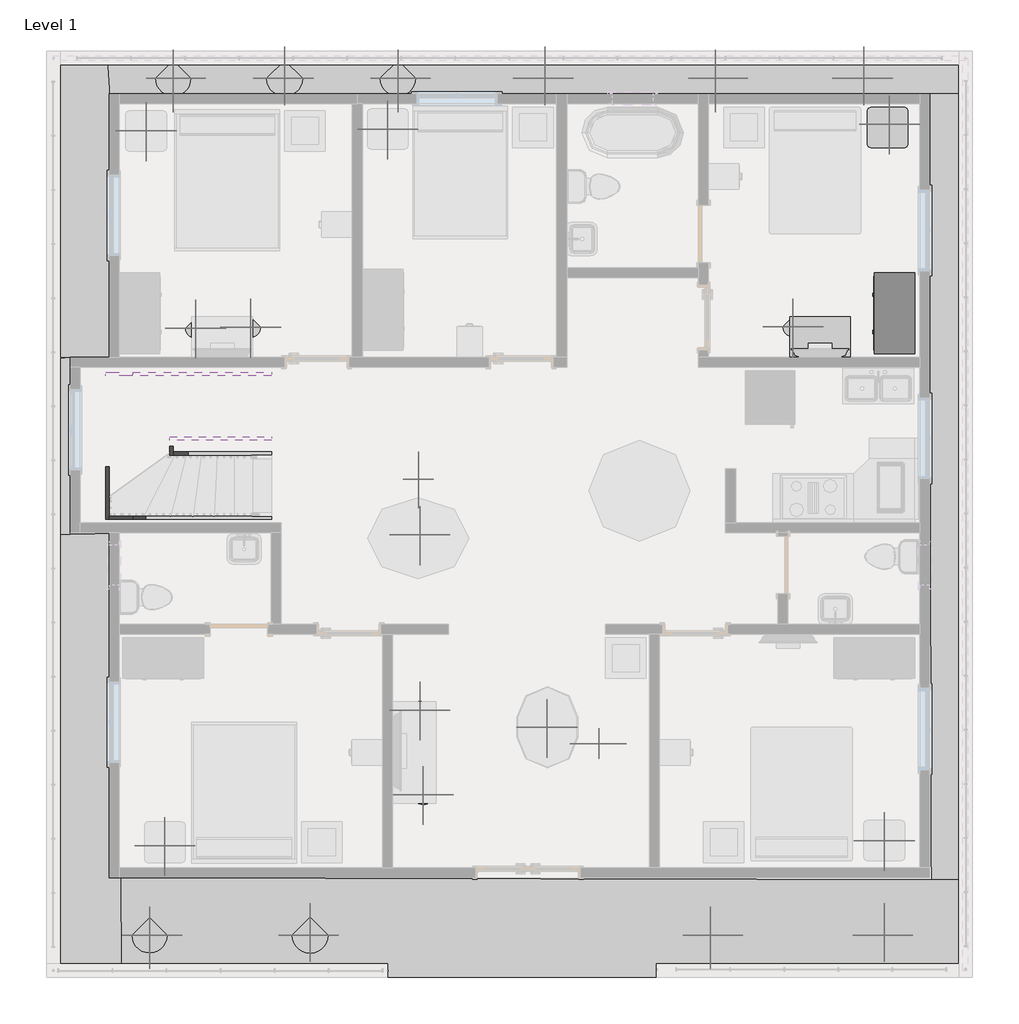
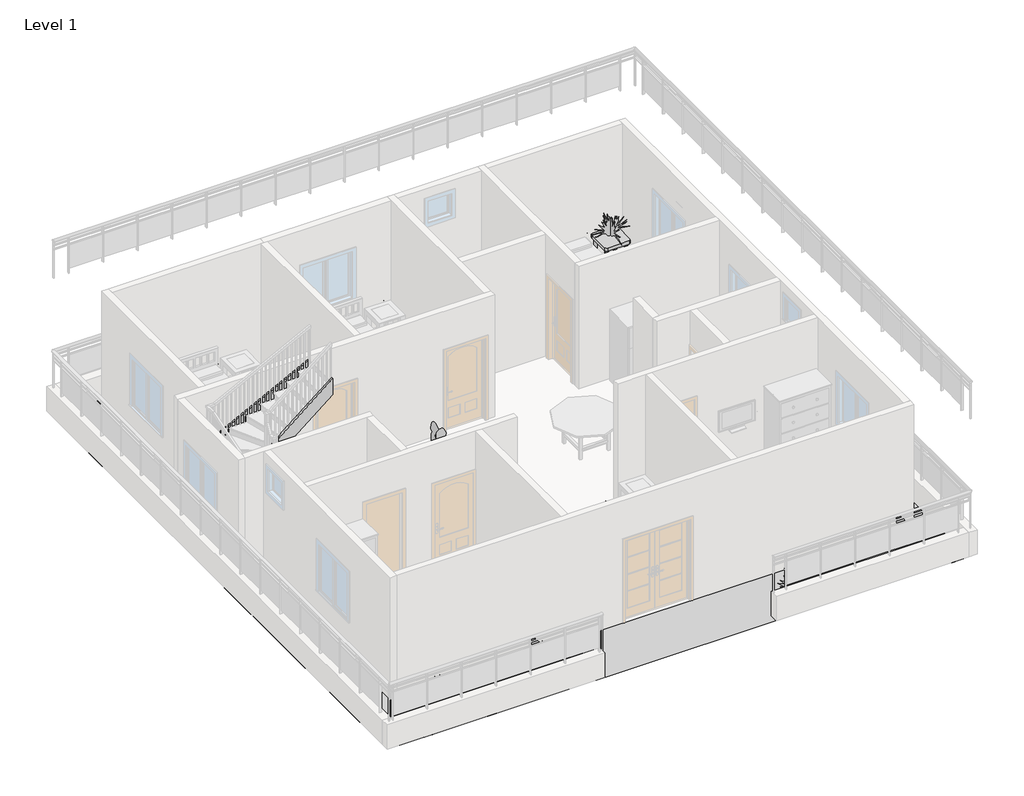
# One storey, part 5 of 5: 22 geographic elements, 8 members, 8 proxies, 3 furniture elements.
"""IFC4 building model written with IfcOpenShell, lengths in millimetres."""

from ifc_helpers import new_model, si_unit, frame, origin, place, context, project, spatial, polyline, outline, extrude, triangles, transform, mapped, element, save
from components import rpc_female_69e001fa, furniture_9fa109b2, furniture_31d08a24, furniture_5341d497, rpc_plant_tropical_55f6ff97, rpc_plant_tropical_agave_1_5_93a2a214, rpc_plant_tropical_jungle_flame_3_9c4808c2

model = new_model("IFC4")

# Units and contexts
model_context = context("Model", 3, world=origin())
ifc_project = project(units=[si_unit("LENGTHUNIT", "METRE", prefix="MILLI")], contexts=[model_context])

# Site, building, storey
site = spatial("IfcSite", under=ifc_project)
building = spatial("IfcBuilding", under=site)
storey = spatial("IfcBuildingStorey", under=building, Name="Level 1", Elevation=0.0)

# Proxies
placement = place(None, origin())
element("IfcBuildingElementProxy", 1, Name="Building Element Proxy", at=placement, inside=storey, context=model_context, shape_type="Tessellation", body=[
    triangles([(-11580.6431305, 14443.7718567, 0.0), (-10674.413562, 14443.7718567, 0.0), (-10640.8435181, 9846.3722443, 0.0), (-11580.6431305, 9837.6390564, 0.0), (-10635.1589813, 13880.7631989, 0.0)], [[1, 4, 5], [1, 5, 2], [5, 4, 3]], closed=False),
])
element("IfcBuildingElementProxy", 2, Name="Building Element Proxy", at=placement, inside=storey, context=model_context, shape_type="Tessellation", body=[
    triangles([(-10640.8435181, 13808.7722443, 0.0), (-10674.3833313, 14240.5714691, 0.0), (2135.3565788, 14240.5714691, 0.0), (2338.5565304, 14228.0826965, 0.0), (2338.5565304, 13813.1347687, 0.0)], [[2, 1, 3], [3, 5, 4], [5, 3, 1]], closed=False),
])
element("IfcBuildingElementProxy", 3, Name="Building Element Proxy", at=placement, inside=storey, context=model_context, shape_type="Tessellation", body=[
    triangles([(1728.9565304, 13808.7722443, 0.0), (2338.5565304, 13786.7387054, 0.0), (2338.5565304, 524.5716871, 0.0), (1729.3105785, 524.5716871, 0.0), (2135.3565788, 13813.3545227, 0.0), (1703.5564819, 13808.7722443, 0.0)], [[6, 4, 1], [1, 4, 2], [6, 1, 5], [1, 2, 5], [2, 4, 3]], closed=False),
])
element("IfcBuildingElementProxy", 4, Name="Building Element Proxy", at=placement, inside=storey, context=model_context, shape_type="Tessellation", body=[
    triangles([(2338.5565304, 524.5716871, 0.0), (2338.5565304, 1993.3553627, 0.0), (-10640.8435181, 2023.1717113, 0.0), (-10535.8080688, 524.5716871, 0.0), (-10617.6030762, 727.7717113, 0.0)], [[3, 5, 4], [4, 1, 2], [4, 2, 3]], closed=False),
])
element("IfcBuildingElementProxy", 5, Name="Building Element Proxy", at=placement, inside=storey, context=model_context, shape_type="Tessellation", body=[
    triangles([(-10488.4435181, 7204.7718567, 0.0), (-11580.6431305, 7176.5578812, 0.0), (-11580.6431305, 524.5716871, 0.0), (-10456.9012573, 524.5716871, 0.0)], [[2, 3, 4], [4, 1, 2]], closed=False),
])
element("IfcBuildingElementProxy", 6, Name="Building Element Proxy", at=placement, inside=storey, context=model_context, shape_type="Tessellation", body=[
    triangles([(-11377.4439056, 9828.7930847, 0.0), (-11377.4439056, 7181.2756165, 0.0), (-11225.0439056, 7204.7718567, 0.0), (-11225.0439056, 9846.3722443, 0.0), (-11231.0167969, 7166.6317429, 0.0)], [[1, 2, 3], [3, 4, 1], [3, 2, 5]], closed=False),
])
rpc_female_shape = rpc_female_69e001fa(model_context)
element("IfcBuildingElementProxy", 7, Name="RPC Female", ObjectType="RPC Female", at=placement, inside=storey, context=model_context, shape_type="MappedRepresentation", body=[
    mapped(rpc_female_shape, transform((-5992.6434666, 7852.4716937, 0.0), x_axis=(1.0, 0.0, 0.0), y_axis=(0.0, 1.0, 0.0), z_axis=(0.0, 0.0, 1.0))),
])
element("IfcBuildingElementProxy", 8, Name="RPC Female", ObjectType="RPC Female", at=placement, inside=storey, context=model_context, shape_type="MappedRepresentation", body=[
    mapped(rpc_female_shape, transform((-3433.5934666, 4041.1791756, 0.0), x_axis=(0.0, -1.0000000000000004, 0.0), y_axis=(1.0000000000000004, 0.0, 0.0), z_axis=(0.0, 0.0, 1.0))),
])

# Furniture
furniture_shape = furniture_9fa109b2(model_context)
element("IfcFurniture", 9, ObjectType="Dresser : 48\" x 72\" x 24\"", at=placement, inside=storey, context=model_context, shape_type="MappedRepresentation", body=[
    mapped(furniture_shape, transform((1533.3194875, 10237.5784339, 0.0), x_axis=(0.0, -1.0000000000000004, 0.0), y_axis=(1.0000000000000004, 0.0, 0.0), z_axis=(0.0, 0.0, 1.0))),
])
furniture_2_shape = furniture_31d08a24(model_context)
element("IfcFurniture", 10, ObjectType="Table-End : 24\" x 24\"", at=placement, inside=storey, context=model_context, shape_type="MappedRepresentation", body=[
    mapped(furniture_2_shape, transform((760.0229031, 13148.3716937, 0.0), x_axis=(1.0, 0.0, 0.0), y_axis=(0.0, 1.0, 0.0), z_axis=(0.0, 0.0, 1.0))),
])
furniture_3_shape = furniture_5341d497(model_context)
element("IfcFurniture", 11, ObjectType="Table-Rectangular : 72\" x 30\"", at=placement, inside=storey, context=model_context, shape_type="MappedRepresentation", body=[
    mapped(furniture_3_shape, transform((52.5565334, 10151.1716937, 0.0), x_axis=(1.0, 0.0, 0.0), y_axis=(0.0, 1.0, 0.0), z_axis=(0.0, 0.0, 1.0))),
])

# Geographic elements
rpc_plant_tropical_shape = rpc_plant_tropical_55f6ff97(model_context)
element("IfcGeographicElement", 12, ObjectType="RPC Plant - Tropical", at=placement, inside=storey, context=model_context, shape_type="MappedRepresentation", body=[
    mapped(rpc_plant_tropical_shape, transform((-10031.2434666, 1159.5716937, 0.0), x_axis=(1.0, 0.0, 0.0), y_axis=(0.0, 1.0, 0.0), z_axis=(0.0, 0.0, 1.0))),
])
element("IfcGeographicElement", 13, ObjectType="RPC Plant - Tropical", at=placement, inside=storey, context=model_context, shape_type="MappedRepresentation", body=[
    mapped(rpc_plant_tropical_shape, transform((-1598.4434666, 1159.5716937, 0.0), x_axis=(1.0, 0.0, 0.0), y_axis=(0.0, 1.0, 0.0), z_axis=(0.0, 0.0, 1.0))),
])
element("IfcGeographicElement", 14, ObjectType="RPC Plant - Tropical", at=placement, inside=storey, context=model_context, shape_type="MappedRepresentation", body=[
    mapped(rpc_plant_tropical_shape, transform((-9675.6434666, 14037.3716937, 0.0), x_axis=(1.0, 0.0, 0.0), y_axis=(0.0, 1.0, 0.0), z_axis=(0.0, 0.0, 1.0))),
])
element("IfcGeographicElement", 15, ObjectType="RPC Plant - Tropical", at=placement, inside=storey, context=model_context, shape_type="MappedRepresentation", body=[
    mapped(rpc_plant_tropical_shape, transform((-6297.4434666, 14037.3716937, 0.0), x_axis=(1.0, 0.0, 0.0), y_axis=(0.0, 1.0, 0.0), z_axis=(0.0, 0.0, 1.0))),
])
element("IfcGeographicElement", 16, ObjectType="RPC Plant - Tropical", at=placement, inside=storey, context=model_context, shape_type="MappedRepresentation", body=[
    mapped(rpc_plant_tropical_shape, transform((-1522.2434666, 14037.3716937, 0.0), x_axis=(1.0, 0.0, 0.0), y_axis=(0.0, 1.0, 0.0), z_axis=(0.0, 0.0, 1.0))),
])
rpc_plant_tropical_agave_1_5_shape = rpc_plant_tropical_agave_1_5_93a2a214(model_context)
element("IfcGeographicElement", 17, ObjectType="RPC Plant - Tropical : Agave - 1.5'", at=placement, inside=storey, context=model_context, shape_type="MappedRepresentation", body=[
    mapped(rpc_plant_tropical_agave_1_5_shape, transform((-10082.0434666, 13249.9716937, 609.6), x_axis=(1.0, 0.0, 0.0), y_axis=(0.0, 1.0, 0.0), z_axis=(0.0, 0.0, 1.0))),
])
element("IfcGeographicElement", 18, ObjectType="RPC Plant - Tropical : Agave - 1.5'", at=placement, inside=storey, context=model_context, shape_type="MappedRepresentation", body=[
    mapped(rpc_plant_tropical_agave_1_5_shape, transform((-6449.8434666, 13275.3716937, 609.6), x_axis=(1.0, 0.0, 0.0), y_axis=(0.0, 1.0, 0.0), z_axis=(0.0, 0.0, 1.0))),
])
element("IfcGeographicElement", 19, ObjectType="RPC Plant - Tropical : Agave - 1.5'", at=placement, inside=storey, context=model_context, shape_type="MappedRepresentation", body=[
    mapped(rpc_plant_tropical_agave_1_5_shape, transform((1093.9565334, 13351.5716937, 609.6), x_axis=(1.0, 0.0, 0.0), y_axis=(0.0, 1.0, 0.0), z_axis=(0.0, 0.0, 1.0))),
])
element("IfcGeographicElement", 20, ObjectType="RPC Plant - Tropical : Agave - 1.5'", at=placement, inside=storey, context=model_context, shape_type="MappedRepresentation", body=[
    mapped(rpc_plant_tropical_agave_1_5_shape, transform((-9802.6434666, 2505.7716937, 609.6), x_axis=(1.0, 0.0, 0.0), y_axis=(0.0, 1.0, 0.0), z_axis=(0.0, 0.0, 1.0))),
])
element("IfcGeographicElement", 21, ObjectType="RPC Plant - Tropical : Agave - 1.5'", at=placement, inside=storey, context=model_context, shape_type="MappedRepresentation", body=[
    mapped(rpc_plant_tropical_agave_1_5_shape, transform((1017.7565334, 2581.9716937, 609.6), x_axis=(1.0, 0.0, 0.0), y_axis=(0.0, 1.0, 0.0), z_axis=(0.0, 0.0, 1.0))),
])
element("IfcGeographicElement", 22, ObjectType="RPC Plant - Tropical : Agave - 1.5'", at=placement, inside=storey, context=model_context, shape_type="MappedRepresentation", body=[
    mapped(rpc_plant_tropical_agave_1_5_shape, transform((-8513.5934666, 10297.2216937, 660.4), x_axis=(1.0, 0.0, 0.0), y_axis=(0.0, 1.0, 0.0), z_axis=(0.0, 0.0, 1.0))),
])
element("IfcGeographicElement", 23, ObjectType="RPC Plant - Tropical : Agave - 1.5'", at=placement, inside=storey, context=model_context, shape_type="MappedRepresentation", body=[
    mapped(rpc_plant_tropical_agave_1_5_shape, transform((-9339.0934666, 10284.5216937, 660.4), x_axis=(1.0, 0.0, 0.0), y_axis=(0.0, 1.0, 0.0), z_axis=(0.0, 0.0, 1.0))),
])
element("IfcGeographicElement", 24, ObjectType="RPC Plant - Tropical : Agave - 1.5'", at=placement, inside=storey, context=model_context, shape_type="MappedRepresentation", body=[
    mapped(rpc_plant_tropical_agave_1_5_shape, transform((-353.8434666, 10303.5716937, 660.4), x_axis=(1.0, 0.0, 0.0), y_axis=(0.0, 1.0, 0.0), z_axis=(0.0, 0.0, 1.0))),
])
element("IfcGeographicElement", 25, ObjectType="RPC Plant - Tropical : Agave - 1.5'", at=placement, inside=storey, context=model_context, shape_type="MappedRepresentation", body=[
    mapped(rpc_plant_tropical_agave_1_5_shape, transform((-4055.8934666, 4283.7716937, 736.6), x_axis=(1.0, 0.0, 0.0), y_axis=(0.0, 1.0, 0.0), z_axis=(0.0, 0.0, 1.0))),
])
element("IfcGeographicElement", 26, ObjectType="RPC Plant - Tropical : Agave - 1.5'", at=placement, inside=storey, context=model_context, shape_type="MappedRepresentation", body=[
    mapped(rpc_plant_tropical_agave_1_5_shape, transform((-5967.2434666, 4541.7958535, 660.4), x_axis=(1.0, 0.0, 0.0), y_axis=(0.0, 1.0, 0.0), z_axis=(0.0, 0.0, 1.0))),
])
element("IfcGeographicElement", 27, ObjectType="RPC Plant - Tropical : Agave - 1.5'", at=placement, inside=storey, context=model_context, shape_type="MappedRepresentation", body=[
    mapped(rpc_plant_tropical_agave_1_5_shape, transform((-5916.4434666, 3271.7958535, 660.4), x_axis=(1.0, 0.0, 0.0), y_axis=(0.0, 1.0, 0.0), z_axis=(0.0, 0.0, 1.0))),
])
element("IfcGeographicElement", 28, ObjectType="RPC Plant - Tropical : Agave - 1.5'", at=placement, inside=storey, context=model_context, shape_type="MappedRepresentation", body=[
    mapped(rpc_plant_tropical_agave_1_5_shape, transform((-5967.2434666, 7179.3716937, 609.6), x_axis=(1.0, 0.0, 0.0), y_axis=(0.0, 1.0, 0.0), z_axis=(0.0, 0.0, 1.0))),
])
rpc_plant_tropical_jungle_flame_3_shape = rpc_plant_tropical_jungle_flame_3_9c4808c2(model_context)
element("IfcGeographicElement", 29, ObjectType="RPC Plant - Tropical : Jungle Flame - 3'", at=placement, inside=storey, context=model_context, shape_type="MappedRepresentation", body=[
    mapped(rpc_plant_tropical_jungle_flame_3_shape, transform((-7618.2434666, 1159.5716937, 0.0), x_axis=(1.0, 0.0, 0.0), y_axis=(0.0, 1.0, 0.0), z_axis=(0.0, 0.0, 1.0))),
])
element("IfcGeographicElement", 30, ObjectType="RPC Plant - Tropical : Jungle Flame - 3'", at=placement, inside=storey, context=model_context, shape_type="MappedRepresentation", body=[
    mapped(rpc_plant_tropical_jungle_flame_3_shape, transform((1017.7565334, 1159.5716937, 0.0), x_axis=(1.0, 0.0, 0.0), y_axis=(0.0, 1.0, 0.0), z_axis=(0.0, 0.0, 1.0))),
])
element("IfcGeographicElement", 31, ObjectType="RPC Plant - Tropical : Jungle Flame - 3'", at=placement, inside=storey, context=model_context, shape_type="MappedRepresentation", body=[
    mapped(rpc_plant_tropical_jungle_flame_3_shape, transform((-7999.2434666, 14037.3716937, 0.0), x_axis=(1.0, 0.0, 0.0), y_axis=(0.0, 1.0, 0.0), z_axis=(0.0, 0.0, 1.0))),
])
element("IfcGeographicElement", 32, ObjectType="RPC Plant - Tropical : Jungle Flame - 3'", at=placement, inside=storey, context=model_context, shape_type="MappedRepresentation", body=[
    mapped(rpc_plant_tropical_jungle_flame_3_shape, transform((-4087.6434666, 14037.3716937, 0.0), x_axis=(1.0, 0.0, 0.0), y_axis=(0.0, 1.0, 0.0), z_axis=(0.0, 0.0, 1.0))),
])
element("IfcGeographicElement", 33, ObjectType="RPC Plant - Tropical : Jungle Flame - 3'", at=placement, inside=storey, context=model_context, shape_type="MappedRepresentation", body=[
    mapped(rpc_plant_tropical_jungle_flame_3_shape, transform((712.9565334, 14037.3716937, 0.0), x_axis=(1.0, 0.0, 0.0), y_axis=(0.0, 1.0, 0.0), z_axis=(0.0, 0.0, 1.0))),
])

# Members
element("IfcMember", 34, ObjectType="Stringer - 2\" Width", at=placement, inside=storey, context=model_context, shape_type="SweptSolid", body=[
    extrude(outline(polyline([(0.0, -8198.7117747), (229.639954, -8198.7117747), (1305.3956453, -10286.1289664), (962.500629, -10286.1289664), (0.0, -8418.4740923), (0.0, -8198.7117747)])), frame((0.0, 7407.9716937, 0.0), z_axis=(0.0, 1.0, 0.0), x_axis=(0.0, 0.0, 1.0)), (0.0, 0.0, 1.0), 50.8),
])
element("IfcMember", 35, ObjectType="Stringer - 2\" Width", at=placement, inside=storey, context=model_context, shape_type="SweptSolid", body=[
    extrude(outline(polyline([(-10286.1289664, 7458.7716937), (-10286.1289664, 7407.9716937), (-10640.8434666, 7407.9716937), (-10640.8434666, 7458.7716937), (-10286.1289664, 7458.7716937)])), frame((0.0, 0.0, 962.500629), z_axis=(0.0, 0.0, 1.0), x_axis=(1.0, 0.0, 0.0)), (0.0, 0.0, 1.0), 342.8950162),
])
element("IfcMember", 36, ObjectType="Stringer - 2\" Width", at=placement, inside=storey, context=model_context, shape_type="SweptSolid", body=[
    extrude(outline(polyline([(7407.9716937, 1000.5956453), (7407.9716937, 1289.0952212), (9529.9915764, 1969.9972697), (9566.9716937, 1969.9972697), (9566.9716937, 1638.9682298), (7577.4941767, 1000.5956453), (7407.9716937, 1000.5956453)])), frame((-10691.6434666, 0.0, 0.0), z_axis=(1.0, 0.0, 0.0), x_axis=(0.0, 1.0, 0.0)), (0.0, 0.0, 1.0), 50.8),
])
element("IfcMember", 37, ObjectType="Stringer - 2\" Width", at=placement, inside=storey, context=model_context, shape_type="SweptSolid", body=[
    extrude(outline(polyline([(-10691.6434666, 9566.9716937), (-10691.6434666, 9617.7716937), (-10286.1289664, 9617.7716937), (-10286.1289664, 9566.9716937), (-10691.6434666, 9566.9716937)])), frame((0.0, 0.0, 1649.8904473), z_axis=(0.0, 0.0, 1.0), x_axis=(1.0, 0.0, 0.0)), (0.0, 0.0, 1.0), 320.1068224),
])
element("IfcMember", 38, ObjectType="Stringer - 2\" Width", at=placement, inside=storey, context=model_context, shape_type="SweptSolid", body=[
    extrude(outline(polyline([(1969.9972697, -10286.1289664), (1649.8904473, -10286.1289664), (2725.6461385, -8198.7117747), (3045.7529609, -8198.7117747), (1969.9972697, -10286.1289664)])), frame((0.0, 9566.9716937, 0.0), z_axis=(0.0, 1.0, 0.0), x_axis=(0.0, 0.0, 1.0)), (0.0, 0.0, 1.0), 50.8),
])
element("IfcMember", 39, ObjectType="Stringer - 2\" Width", at=placement, inside=storey, context=model_context, shape_type="SweptSolid", body=[
    extrude(outline(polyline([(0.0, -8198.7117747), (176.1764461, -8198.7117747), (1380.418648, -9675.6434666), (987.1410923, -9675.6434666), (0.0, -8464.9734193), (0.0, -8198.7117747)])), frame((0.0, 8373.1716937, 0.0), z_axis=(0.0, 1.0, 0.0), x_axis=(0.0, 0.0, 1.0)), (0.0, 0.0, 1.0), 50.8),
])
element("IfcMember", 40, ObjectType="Stringer - 2\" Width", at=placement, inside=storey, context=model_context, shape_type="SweptSolid", body=[
    extrude(outline(polyline([(8373.1716937, 1028.5617647), (8373.1716937, 1573.2682978), (8579.8088111, 1926.1409689), (8601.7716937, 1926.1409689), (8601.7716937, 1360.465107), (8407.413911, 1028.5617647), (8373.1716937, 1028.5617647)])), frame((-9726.4434666, 0.0, 0.0), z_axis=(1.0, 0.0, 0.0), x_axis=(0.0, 1.0, 0.0)), (0.0, 0.0, 1.0), 50.8),
])
element("IfcMember", 41, ObjectType="Stringer - 2\" Width", at=placement, inside=storey, context=model_context, shape_type="SweptSolid", body=[
    extrude(outline(polyline([(1926.1409689, -9726.4434666), (1532.8634131, -9726.4434666), (2778.5262875, -8198.7117747), (3171.8038432, -8198.7117747), (1926.1409689, -9726.4434666)])), frame((0.0, 8601.7716937, 0.0), z_axis=(0.0, 1.0, 0.0), x_axis=(0.0, 0.0, 1.0)), (0.0, 0.0, 1.0), 50.8),
])

save(model, "model.ifc")

# Revit data of these elements
# Type "RPC Female"
#   built-in parameter 1005195 = "RPC-8-FXA2-QQQ0-UGV2-6"
#   Height = 0
# Type "Dresser : 48\" x 72\" x 24\""
#   Assembly Code = "E2020200"
#   Depth = 2' - 0"
#   Height = 6' - 0"
#   Width = 4' - 0"
#   Dresser Material = Wood - Teak
#   Drawer Material = Wood - Teak
#   Knob Material = Cherry
#   Default Elevation = 0
# Type "Table-End : 24\" x 24\""
#   Assembly Code = "E2020200"
#   Height = 2' - 0"
#   Length = 2' - 0"
#   Width = 2' - 0"
#   Base Material = Birch
#   Top Material = Laminate, Ivory, Matte
#   Default Elevation = 0
# Type "Table-Rectangular : 72\" x 30\""
#   Assembly Code = "E2020200"
#   Height = 2' - 2"
#   Length = 3' - 0"
#   Width = 2' - 0"
#   Base Material = Birch
#   Top Material = Birch
#   Default Elevation = 0
# Type "RPC Plant - Tropical"
#   built-in parameter 1005198 = "{2, 15},{39, RPC-16-FWM5-GM7X-C67P-4000-ST1L-LVER-AU},{1, 0},{1, 0},{2, 13},{1, 8},{5, Color},{1, 0},{1, 0},{3, 0.8},{3, 0.8},{3, 0.8},{1, 8},{7, BBoxMin},{1, 0},{1, 0},{1, 0},{1, 0},{1, 0},{1, 8},{7, BBoxMax},{1, 0},{1, 0},{1, 0},{1, 0},{1, 0},{2, 11},{9, RPCTypeId},{1, 0},{1, 0},{39, RPC-16-FWM5-GM7X-C67P-4000-ST1L-LVER-AU},{1, 6},{14, RPCPlantHeight},{1, 0},{1, 0},{1, 3},{2, 11},{7, keyword},{1, 0},{1, 0},{35, :RPCs:Shrubs [General]:Geometry:RPC},{2, 11},{8, category},{1, 0},{1, 0},{16, Shrubs [General]},{2, 11},{12, LocalizedUID},{1, 0},{1, 0},{10, Crane Lily},{2, 14},{6, Height},{1, 0},{1, 0},{1, 3},{1, 2},{16, Cast Reflections},{1, 0},{1, 0},{1, 0},{1, 2},{12, Cast Shadows},{1, 0},{1, 0},{1, 1},{1, 2},{9, Lock View},{1, 0},{1, 0},{1, 0},{1, 4},{5, ViewC},{1, 0},{1, 0},{1, 0},{21, assetlibrary_base.fbx},{1, 5},"
#   built-in parameter 1005195 = "RPC-16-FWM5-GM7X-C67P-4000-ST1L-LVER-AU"
#   Assembly Code = "G2050500"
#   Height = 3' - 0"
#   Default Elevation = 0
# Type "RPC Plant - Tropical : Agave - 1.5'"
#   built-in parameter 1005198 = "{2, 15},{39, RPC-16-G1GJ-63FX-7K5P-N000-ST1L-LVER-AU},{1, 0},{1, 0},{2, 13},{1, 8},{5, Color},{1, 0},{1, 0},{3, 0.8},{3, 0.8},{3, 0.8},{1, 8},{7, BBoxMin},{1, 0},{1, 0},{1, 0},{1, 0},{1, 0},{1, 8},{7, BBoxMax},{1, 0},{1, 0},{1, 0},{1, 0},{1, 0},{2, 11},{9, RPCTypeId},{1, 0},{1, 0},{39, RPC-16-G1GJ-63FX-7K5P-N000-ST1L-LVER-AU},{1, 6},{14, RPCPlantHeight},{1, 0},{1, 0},{3, 1.5},{2, 11},{7, keyword},{1, 0},{1, 0},{35, :RPCs:Plants [General]:Geometry:RPC},{2, 11},{8, category},{1, 0},{1, 0},{16, Plants [General]},{2, 11},{12, LocalizedUID},{1, 0},{1, 0},{5, Agave},{2, 14},{6, Height},{1, 0},{1, 0},{3, 1.5},{1, 2},{16, Cast Reflections},{1, 0},{1, 0},{1, 0},{1, 2},{12, Cast Shadows},{1, 0},{1, 0},{1, 1},{1, 2},{9, Lock View},{1, 0},{1, 0},{1, 0},{1, 4},{5, ViewC},{1, 0},{1, 0},{1, 0},{21, assetlibrary_base.fbx},{1, 5},"
#   built-in parameter 1005195 = "RPC-16-G1GJ-63FX-7K5P-N000-ST1L-LVER-AU"
#   Type Comments = "Agave"
#   Assembly Code = "G2050500"
#   Height = 1' - 6"
#   Default Elevation = 0
# Type "RPC Plant - Tropical : Jungle Flame - 3'"
#   built-in parameter 1005198 = "{2, 15},{39, RPC-16-FUVJ-JWG0-MWGK-8000-ST1L-LVER-AU},{1, 0},{1, 0},{2, 13},{1, 8},{5, Color},{1, 0},{1, 0},{3, 0.8},{3, 0.8},{3, 0.8},{1, 8},{7, BBoxMin},{1, 0},{1, 0},{1, 0},{1, 0},{1, 0},{1, 8},{7, BBoxMax},{1, 0},{1, 0},{1, 0},{1, 0},{1, 0},{2, 11},{9, RPCTypeId},{1, 0},{1, 0},{39, RPC-16-FUVJ-JWG0-MWGK-8000-ST1L-LVER-AU},{1, 6},{14, RPCPlantHeight},{1, 0},{1, 0},{1, 3},{2, 11},{7, keyword},{1, 0},{1, 0},{35, :RPCs:Shrubs [General]:Geometry:RPC},{2, 11},{8, category},{1, 0},{1, 0},{16, Shrubs [General]},{2, 11},{12, LocalizedUID},{1, 0},{1, 0},{12, Jungle Flame},{2, 14},{6, Height},{1, 0},{1, 0},{1, 3},{1, 2},{16, Cast Reflections},{1, 0},{1, 0},{1, 0},{1, 2},{12, Cast Shadows},{1, 0},{1, 0},{1, 1},{1, 2},{9, Lock View},{1, 0},{1, 0},{1, 0},{1, 4},{5, ViewC},{1, 0},{1, 0},{1, 0},{21, assetlibrary_base.fbx},{1, 5},"
#   built-in parameter 1005195 = "RPC-16-FUVJ-JWG0-MWGK-8000-ST1L-LVER-AU"
#   Type Comments = "Jungle Flame"
#   Assembly Code = "G2050500"
#   Height = 3' - 0"
#   Default Elevation = 0
# Elements 1, 2, 3, 4, 5, 6 (IfcBuildingElementProxy)
#   Material = Plant
#   Phase Created = New Construction
# Elements 7, 8 (IfcBuildingElementProxy, "RPC Female")
#   Phase Created = New Construction
# Element 9 (IfcFurniture, "Dresser : 48\" x 72\" x 24\"")
#   Phase Created = New Construction
#   Materials on its faces: "Laminate, Ivory, Matte", "Cherry", "Wood - Teak"
# Element 10 (IfcFurniture, "Table-End : 24\" x 24\"")
#   Phase Created = New Construction
#   Materials on its faces: "Laminate, Ivory, Matte", "Birch"
# Element 11 (IfcFurniture, "Table-Rectangular : 72\" x 30\"")
#   Phase Created = New Construction
#   Materials on its faces: "Birch"
# Elements 12, 13, 14, 15, 16 (IfcGeographicElement, "RPC Plant - Tropical")
#   Phase Created = New Construction
# Elements 17, 18, 19, 20, 21, 22, 23, 24, 25, 26, 27, 28 (IfcGeographicElement, "RPC Plant - Tropical : Agave - 1.5'")
#   Phase Created = New Construction
# Elements 29, 30, 31, 32, 33 (IfcGeographicElement, "RPC Plant - Tropical : Jungle Flame - 3'")
#   Phase Created = New Construction
# Elements 34, 35, 36, 37, 38, 39, 40, 41 (IfcMember, "Stringer - 2\" Width")
#   Phase Created = New Construction
# Materials
#   "Wood - Teak": class "Wood", colour RGB 145 112 90, transparency 0
#   "Cherry": class "Wood", colour RGB 226 177 128, transparency 0, Description = "Prunus Serotina", Cost = 0
#   "Birch": class "Wood", colour RGB 224 178 126, transparency 0, Description = "Betula Alleghaniensis", Cost = 0
#   "Laminate, Ivory, Matte": class "Plastic", colour RGB 247 247 239, transparency 0, Description = "Plastic Laminate - Ivory, Matte", Cost = 0
#   "Plant": class "Generic", colour RGB 0 0 0, transparency 0, Description = "physical material", Cost = 0
